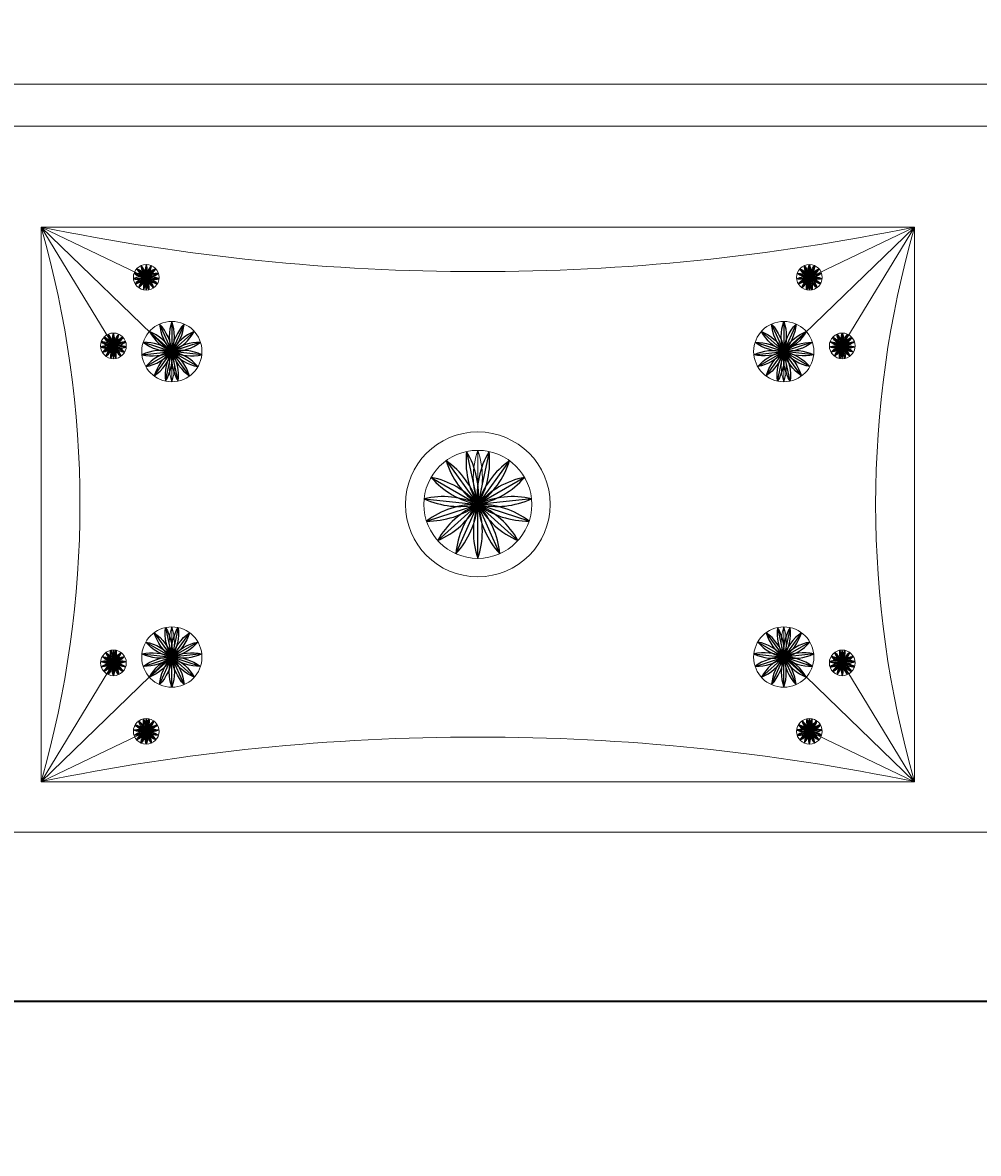
# Model space of a CAD drawing. Units: inches. Extents: x -61 to 1599, y -1316 to 257.
# Tile 5 of 204: x 123 to 149, y -1211 to -1180. Entities that reach past the tile are written whole.
import ezdxf

# ---------------------------------------------------------------- set-up
doc = ezdxf.new("R2010")
doc.units = ezdxf.units.IN
doc.header["$MEASUREMENT"] = 0
for name, color, linetype, lineweight in [('A-ANNO-DIMS', 2, 'Continuous', 18), ('FURNITURE', 83, 'Continuous', 18), ('WALLS', 4, 'Continuous', 35)]:
    doc.layers.add(name, color=color, linetype=linetype, lineweight=lineweight)
doc.layers.add('LT', color=8, linetype='Continuous')
doc.styles.get("Standard").update_dxf_attribs({"font": 'arial.ttf'})
doc.dimstyles.get("Standard").update_dxf_attribs({"dimtxt": 0.18, "dimasz": 0.18, "dimexe": 0.18, "dimexo": 0.0625, "dimgap": 0.09, "dimtad": 0, "dimtih": 1, "dimtoh": 1, "dimdec": 0, "dimzin": 0, "dimdsep": 46, "dimlunit": 3, "dimtxsty": 'Standard', "dimcen": 0.09, "dimadec": 0, "dimazin": 0, "dimtfac": 1, "dimtdec": 0, "dimtofl": 0, "dimtmove": 0, "dimatfit": 3, "dimfxl": 1, "dimtolj": 1, "dimtzin": 0, "dimarcsym": 0})

# ---------------------------------------------------------------- blocks, each defined once
blk = doc.blocks.new('*U15')
at = {"layer": 'LT'}
blk.add_line((0, 0.175), (0, -0.175), dxfattribs=at)
for centre, start, end in [((0.509, 0), 160.9983, 199.0017), ((-0.509, 0), 340.9983, 19.0017)]:
    blk.add_arc(centre, 0.539, start, end, dxfattribs=at)
blk = doc.blocks.new('*U16')
at = {"layer": 'LT', "transparency": 16777216}
for p, rotation in [((-66.605, -18.692), 48.00000000000001), ((-66.546, -18.649), 24), ((-66.404, -18.649), 336.0000000000001), ((-66.345, -18.692), 312), ((-66.649, -18.828), 96), ((-66.642, -18.755), 72), ((-66.627, -18.897), 120), ((-66.578, -18.951), 144), ((-66.512, -18.981), 168.0000000000001), ((-66.439, -18.981), 192), ((-66.372, -18.951), 216), ((-66.323, -18.897), 240), ((-66.308, -18.755), 288.0000000000001), ((-66.301, -18.828), 264)]:
    blk.add_blockref('*U15', p, dxfattribs=dict(at, rotation=rotation))
blk.add_blockref('*U15', (-66.475, -18.634), dxfattribs=at)
blk = doc.blocks.new('*U45')
at = {"layer": 'LT'}
blk.add_line((0, 0.175), (0, -0.175), dxfattribs=at)
for centre, start, end in [((0.509, 0), 160.9983, 199.0017), ((-0.509, 0), 340.9983, 19.0017)]:
    blk.add_arc(centre, 0.539, start, end, dxfattribs=at)
blk = doc.blocks.new('*U46')
at = {"layer": 'LT', "transparency": 16777216}
for p, rotation in [((-66.605, -18.692), 48.00000000000001), ((-66.546, -18.649), 24), ((-66.404, -18.649), 336.0000000000001), ((-66.345, -18.692), 312), ((-66.649, -18.828), 96), ((-66.642, -18.755), 72), ((-66.627, -18.897), 120), ((-66.578, -18.951), 144), ((-66.512, -18.981), 168.0000000000001), ((-66.439, -18.981), 192), ((-66.372, -18.951), 216), ((-66.323, -18.897), 240), ((-66.308, -18.755), 288.0000000000001), ((-66.301, -18.828), 264)]:
    blk.add_blockref('*U45', p, dxfattribs=dict(at, rotation=rotation))
blk.add_blockref('*U45', (-66.475, -18.634), dxfattribs=at)
blk = doc.blocks.new('*U9')
at = {"layer": 'LT'}
blk.add_line((0, 0.175), (0, -0.175), dxfattribs=at)
for centre, start, end in [((0.509, 0), 160.9983, 199.0017), ((-0.509, 0), 340.9983, 19.0017)]:
    blk.add_arc(centre, 0.539, start, end, dxfattribs=at)
blk = doc.blocks.new('*U10')
at = {"layer": 'LT', "transparency": 16777216}
for p, rotation in [((-66.605, -18.692), 48.00000000000001), ((-66.546, -18.649), 24), ((-66.404, -18.649), 336.0000000000001), ((-66.345, -18.692), 312), ((-66.649, -18.828), 96), ((-66.642, -18.755), 72), ((-66.627, -18.897), 120), ((-66.578, -18.951), 144), ((-66.512, -18.981), 168.0000000000001), ((-66.439, -18.981), 192), ((-66.372, -18.951), 216), ((-66.323, -18.897), 240), ((-66.308, -18.755), 288.0000000000001), ((-66.301, -18.828), 264)]:
    blk.add_blockref('*U9', p, dxfattribs=dict(at, rotation=rotation))
blk.add_blockref('*U9', (-66.475, -18.634), dxfattribs=at)
blk = doc.blocks.new('*U39')
at = {"layer": 'LT'}
blk.add_line((0, 0.175), (0, -0.175), dxfattribs=at)
for centre, start, end in [((0.509, 0), 160.9983, 199.0017), ((-0.509, 0), 340.9983, 19.0017)]:
    blk.add_arc(centre, 0.539, start, end, dxfattribs=at)
blk = doc.blocks.new('*U40')
at = {"layer": 'LT', "transparency": 16777216}
for p, rotation in [((-66.605, -18.692), 48.00000000000001), ((-66.546, -18.649), 24), ((-66.404, -18.649), 336.0000000000001), ((-66.345, -18.692), 312), ((-66.649, -18.828), 96), ((-66.642, -18.755), 72), ((-66.627, -18.897), 120), ((-66.578, -18.951), 144), ((-66.512, -18.981), 168.0000000000001), ((-66.439, -18.981), 192), ((-66.372, -18.951), 216), ((-66.323, -18.897), 240), ((-66.308, -18.755), 288.0000000000001), ((-66.301, -18.828), 264)]:
    blk.add_blockref('*U39', p, dxfattribs=dict(at, rotation=rotation))
blk.add_blockref('*U39', (-66.475, -18.634), dxfattribs=at)
blk = doc.blocks.new('*U17')
at = {"layer": 'LT'}
blk.add_line((0, 0.412), (0, -0.412), dxfattribs=at)
for centre, start, end in [((1.198, 0), 160.9983, 199.0017), ((-1.198, 0), 340.9983, 19.0017)]:
    blk.add_arc(centre, 1.267, start, end, dxfattribs=at)
blk = doc.blocks.new('*U18')
at = {"layer": 'LT', "transparency": 16777216}
for p, rotation in [((-156.501, -43.858), 24), ((-156.165, -43.858), 336.0000000000001), ((-156.725, -44.108), 72), ((-156.639, -43.959), 48.00000000000001), ((-156.027, -43.959), 312), ((-155.941, -44.108), 288.0000000000001), ((-156.743, -44.278), 96), ((-156.69, -44.441), 120), ((-156.575, -44.569), 144), ((-156.419, -44.639), 168), ((-156.247, -44.639), 192), ((-156.091, -44.569), 216), ((-155.976, -44.441), 240), ((-155.923, -44.278), 264)]:
    blk.add_blockref('*U17', p, dxfattribs=dict(at, rotation=rotation))
blk.add_blockref('*U17', (-156.333, -43.823), dxfattribs=at)
blk = doc.blocks.new('*U33')
at = {"layer": 'LT'}
blk.add_line((0, 0.412), (0, -0.412), dxfattribs=at)
for centre, start, end in [((1.198, 0), 160.9983, 199.0017), ((-1.198, 0), 340.9983, 19.0017)]:
    blk.add_arc(centre, 1.267, start, end, dxfattribs=at)
blk = doc.blocks.new('*U34')
at = {"layer": 'LT', "transparency": 16777216}
for p, rotation in [((-156.501, -43.858), 24), ((-156.165, -43.858), 336.0000000000001), ((-156.725, -44.108), 72), ((-156.639, -43.959), 48.00000000000001), ((-156.027, -43.959), 312), ((-155.941, -44.108), 288.0000000000001), ((-156.743, -44.278), 96), ((-156.69, -44.441), 120), ((-156.575, -44.569), 144), ((-156.419, -44.639), 168), ((-156.247, -44.639), 192), ((-156.091, -44.569), 216), ((-155.976, -44.441), 240), ((-155.923, -44.278), 264)]:
    blk.add_blockref('*U33', p, dxfattribs=dict(at, rotation=rotation))
blk.add_blockref('*U33', (-156.333, -43.823), dxfattribs=at)
blk = doc.blocks.new('*U11')
at = {"layer": 'LT'}
blk.add_line((0, 0.739), (0, -0.739), dxfattribs=at)
for centre, start, end in [((2.147, 0), 160.9983, 199.0017), ((-2.147, 0), 340.9983, 19.0017)]:
    blk.add_arc(centre, 2.27, start, end, dxfattribs=at)
blk = doc.blocks.new('*U12')
at = {"layer": 'LT', "transparency": 16777216}
for p, rotation in [((-280.542, -78.621), 23.99999999999999), ((-279.941, -78.621), 336.0000000000001), ((-280.791, -78.801), 48.00000000000001), ((-279.692, -78.801), 312), ((-280.945, -79.067), 72), ((-279.539, -79.067), 288.0000000000001), ((-280.977, -79.373), 96), ((-280.882, -79.665), 120), ((-279.602, -79.665), 240), ((-279.507, -79.373), 264), ((-280.676, -79.894), 144), ((-280.395, -80.019), 168), ((-280.088, -80.019), 191.9999999999999), ((-279.807, -79.894), 216)]:
    blk.add_blockref('*U11', p, dxfattribs=dict(at, rotation=rotation))
blk.add_blockref('*U11', (-280.242, -78.557), dxfattribs=at)
blk = doc.blocks.new('*U28')
at = {"layer": 'LT'}
blk.add_line((0, 0.412), (0, -0.412), dxfattribs=at)
for centre, start, end in [((1.198, 0), 160.9983, 199.0017), ((-1.198, 0), 340.9983, 19.0017)]:
    blk.add_arc(centre, 1.267, start, end, dxfattribs=at)
blk = doc.blocks.new('*U44')
at = {"layer": 'LT', "transparency": 16777216}
for p, rotation in [((-156.501, -43.858), 24), ((-156.165, -43.858), 336.0000000000001), ((-156.725, -44.108), 72), ((-156.639, -43.959), 48.00000000000001), ((-156.027, -43.959), 312), ((-155.941, -44.108), 288.0000000000001), ((-156.743, -44.278), 96), ((-156.69, -44.441), 120), ((-156.575, -44.569), 144), ((-156.419, -44.639), 168), ((-156.247, -44.639), 192), ((-156.091, -44.569), 216), ((-155.976, -44.441), 240), ((-155.923, -44.278), 264)]:
    blk.add_blockref('*U28', p, dxfattribs=dict(at, rotation=rotation))
blk.add_blockref('*U28', (-156.333, -43.823), dxfattribs=at)
blk = doc.blocks.new('*U13')
at = {"layer": 'LT'}
blk.add_line((0, 0.412), (0, -0.412), dxfattribs=at)
for centre, start, end in [((1.198, 0), 160.9983, 199.0017), ((-1.198, 0), 340.9983, 19.0017)]:
    blk.add_arc(centre, 1.267, start, end, dxfattribs=at)
blk = doc.blocks.new('*U14')
at = {"layer": 'LT', "transparency": 16777216}
for p, rotation in [((-156.501, -43.858), 24), ((-156.165, -43.858), 336.0000000000001), ((-156.725, -44.108), 72), ((-156.639, -43.959), 48.00000000000001), ((-156.027, -43.959), 312), ((-155.941, -44.108), 288.0000000000001), ((-156.743, -44.278), 96), ((-156.69, -44.441), 120), ((-156.575, -44.569), 144), ((-156.419, -44.639), 168), ((-156.247, -44.639), 192), ((-156.091, -44.569), 216), ((-155.976, -44.441), 240), ((-155.923, -44.278), 264)]:
    blk.add_blockref('*U13', p, dxfattribs=dict(at, rotation=rotation))
blk.add_blockref('*U13', (-156.333, -43.823), dxfattribs=at)
blk = doc.blocks.new('*U19')
at = {"layer": 'LT'}
blk.add_line((0, 0.175), (0, -0.175), dxfattribs=at)
for centre, start, end in [((0.509, 0), 160.9983, 199.0017), ((-0.509, 0), 340.9983, 19.0017)]:
    blk.add_arc(centre, 0.539, start, end, dxfattribs=at)
blk = doc.blocks.new('*U6')
at = {"layer": 'LT', "transparency": 16777216}
for p, rotation in [((-66.605, -18.692), 48.00000000000001), ((-66.546, -18.649), 24), ((-66.404, -18.649), 336.0000000000001), ((-66.345, -18.692), 312), ((-66.649, -18.828), 96), ((-66.642, -18.755), 72), ((-66.627, -18.897), 120), ((-66.578, -18.951), 144), ((-66.512, -18.981), 168.0000000000001), ((-66.439, -18.981), 192), ((-66.372, -18.951), 216), ((-66.323, -18.897), 240), ((-66.308, -18.755), 288.0000000000001), ((-66.301, -18.828), 264)]:
    blk.add_blockref('*U19', p, dxfattribs=dict(at, rotation=rotation))
blk.add_blockref('*U19', (-66.475, -18.634), dxfattribs=at)
blk = doc.blocks.new('*U35')
at = {"layer": 'LT'}
blk.add_line((0, 0.175), (0, -0.175), dxfattribs=at)
for centre, start, end in [((0.509, 0), 160.9983, 199.0017), ((-0.509, 0), 340.9983, 19.0017)]:
    blk.add_arc(centre, 0.539, start, end, dxfattribs=at)
blk = doc.blocks.new('*U36')
at = {"layer": 'LT', "transparency": 16777216}
for p, rotation in [((-66.605, -18.692), 48.00000000000001), ((-66.546, -18.649), 24), ((-66.404, -18.649), 336.0000000000001), ((-66.345, -18.692), 312), ((-66.649, -18.828), 96), ((-66.642, -18.755), 72), ((-66.627, -18.897), 120), ((-66.578, -18.951), 144), ((-66.512, -18.981), 168.0000000000001), ((-66.439, -18.981), 192), ((-66.372, -18.951), 216), ((-66.323, -18.897), 240), ((-66.308, -18.755), 288.0000000000001), ((-66.301, -18.828), 264)]:
    blk.add_blockref('*U35', p, dxfattribs=dict(at, rotation=rotation))
blk.add_blockref('*U35', (-66.475, -18.634), dxfattribs=at)
blk = doc.blocks.new('*U7')
at = {"layer": 'LT'}
blk.add_line((0, 0.175), (0, -0.175), dxfattribs=at)
for centre, start, end in [((0.509, 0), 160.9983, 199.0017), ((-0.509, 0), 340.9983, 19.0017)]:
    blk.add_arc(centre, 0.539, start, end, dxfattribs=at)
blk = doc.blocks.new('*U8')
at = {"layer": 'LT', "transparency": 16777216}
for p, rotation in [((-66.605, -18.692), 48.00000000000001), ((-66.546, -18.649), 24), ((-66.404, -18.649), 336.0000000000001), ((-66.345, -18.692), 312), ((-66.649, -18.828), 96), ((-66.642, -18.755), 72), ((-66.627, -18.897), 120), ((-66.578, -18.951), 144), ((-66.512, -18.981), 168.0000000000001), ((-66.439, -18.981), 192), ((-66.372, -18.951), 216), ((-66.323, -18.897), 240), ((-66.308, -18.755), 288.0000000000001), ((-66.301, -18.828), 264)]:
    blk.add_blockref('*U7', p, dxfattribs=dict(at, rotation=rotation))
blk.add_blockref('*U7', (-66.475, -18.634), dxfattribs=at)
blk = doc.blocks.new('*U37')
at = {"layer": 'LT'}
blk.add_line((0, 0.175), (0, -0.175), dxfattribs=at)
for centre, start, end in [((0.509, 0), 160.9983, 199.0017), ((-0.509, 0), 340.9983, 19.0017)]:
    blk.add_arc(centre, 0.539, start, end, dxfattribs=at)
blk = doc.blocks.new('*U38')
at = {"layer": 'LT', "transparency": 16777216}
for p, rotation in [((-66.605, -18.692), 48.00000000000001), ((-66.546, -18.649), 24), ((-66.404, -18.649), 336.0000000000001), ((-66.345, -18.692), 312), ((-66.649, -18.828), 96), ((-66.642, -18.755), 72), ((-66.627, -18.897), 120), ((-66.578, -18.951), 144), ((-66.512, -18.981), 168.0000000000001), ((-66.439, -18.981), 192), ((-66.372, -18.951), 216), ((-66.323, -18.897), 240), ((-66.308, -18.755), 288.0000000000001), ((-66.301, -18.828), 264)]:
    blk.add_blockref('*U37', p, dxfattribs=dict(at, rotation=rotation))
blk.add_blockref('*U37', (-66.475, -18.634), dxfattribs=at)
blk = doc.blocks.new('BED-DOUBLE')
for p, q in [((1.272, 20.467), (70.263, 20.467)), ((1.272, 19.317), (70.263, 19.317)), ((10.471, 1.379), (10.471, 16.557)), ((34.388, 16.557), (10.471, 16.557)), ((10.471, 16.557), (13.35, 15.18)), ((10.471, 16.557), (14.039, 13.107)), ((10.471, 16.557), (12.454, 13.305)), ((34.388, 16.557), (30.82, 13.107)), ((34.388, 16.557), (31.508, 15.18)), ((34.388, 16.557), (32.405, 13.305)), ((13.35, 15.18), (13.35, 14.829)), ((31.508, 15.18), (31.508, 14.829)), ((12.454, 13.305), (12.454, 12.955)), ((14.052, 13.149), (14.052, 12.324)), ((30.806, 13.149), (30.806, 12.324)), ((32.405, 13.305), (32.405, 12.955)), ((22.429, 8.968), (22.429, 10.447)), ((14.052, 4.788), (14.052, 5.613)), ((30.806, 4.788), (30.806, 5.613)), ((12.454, 4.631), (12.454, 4.982)), ((32.405, 4.631), (32.405, 4.982)), ((10.471, 1.379), (14.039, 4.83)), ((34.388, 1.379), (30.82, 4.83)), ((10.471, 1.379), (12.454, 4.631)), ((34.388, 1.379), (32.405, 4.631)), ((13.35, 2.756), (13.35, 3.107)), ((31.508, 2.756), (31.508, 3.107)), ((10.471, 1.379), (13.35, 2.756)), ((34.388, 1.379), (31.508, 2.756)), ((34.388, 1.379), (34.388, 1.379))]:
    blk.add_line(p, q)
for points in [[(1.272, 88.537), (1.272, 3.449, 0.414214), (4.722, 0), (66.813, 0, 0.414214), (70.263, 3.449), (70.263, 88.537, 0.414214), (66.813, 91.987), (4.722, 91.987, 0.414214)], [(13.35, 15.18, 0.167358), (13.35, 14.829, 0.167358)], [(12.454, 13.305, 0.167358), (12.454, 12.955, 0.167358)], [(14.052, 13.149, 0.167358), (14.052, 12.324, 0.167358)], [(30.806, 12.324, 0.167358), (30.806, 13.149, 0.167358)], [(32.405, 12.955, 0.167358), (32.405, 13.305, 0.167358)], [(22.429, 8.968, 0.167358), (22.429, 10.447, 0.167358)], [(14.052, 5.613, 0.167358), (14.052, 4.788, 0.167358)], [(30.806, 4.788, 0.167358), (30.806, 5.613, 0.167358)], [(12.454, 4.982, 0.167358), (12.454, 4.631, 0.167358)], [(32.405, 4.631, 0.167358), (32.405, 4.982, 0.167358)], [(13.35, 3.107, 0.167358), (13.35, 2.756, 0.167358)], [(31.508, 2.756, 0.167358), (31.508, 3.107, 0.167358)]]:
    blk.add_lwpolyline(points, format="xyb", close=True)
blk.add_lwpolyline([(34.388, 16.557), (34.388, 1.379), (10.471, 1.379), (10.471, 16.557), (34.388, 16.557), (34.388, 1.379), (10.471, 1.379)])
for centre, radius in [((13.35, 15.18), 0.351), ((31.508, 15.18), 0.351), ((14.052, 13.149), 0.825), ((30.806, 13.149), 0.825), ((12.454, 13.305), 0.351), ((32.405, 13.305), 0.351), ((22.429, 8.968), 1.982), ((22.429, 8.968), 1.478), ((14.052, 4.788), 0.825), ((30.806, 4.788), 0.825), ((12.454, 4.631), 0.351), ((32.405, 4.631), 0.351), ((13.35, 2.756), 0.351), ((31.508, 2.756), 0.351)]:
    blk.add_circle(centre, radius)
for centre, radius, start, end in [((-16.003, 8.968), 27.54, 344.0046, 15.9954), ((22.429, 74.54), 59.203, 258.34678, 281.65322), ((60.861, 8.968), 27.54, 164.0046, 195.9954), ((32.017, 15.005), 0.539, 160.9983, 199.0017), ((30.999, 15.005), 0.539, 340.9983, 19.0017), ((22.429, -56.603), 59.203, 78.34678, 101.65322)]:
    blk.add_arc(centre, radius, start, end)
for name, p in [('*U40', (79.825, 33.99)), ('*U34', (170.385, 57.384)), ('*U46', (78.929, 32.115))]:
    blk.add_blockref(name, p)
at = {"extrusion": (0, 0, -1), "zscale": -1}
for name, p in [('*U36', (34.967, 33.99)), ('*U14', (125.527, 57.384)), ('*U38', (34.07, 32.115))]:
    blk.add_blockref(name, p, dxfattribs=at)
at = {"rotation": 180}
for name, p in [('*U12', (-257.812, -70.328)), ('*U44', (-125.527, -39.447)), ('*U8', (-34.07, -14.178)), ('*U6', (-34.967, -16.053))]:
    blk.add_blockref(name, p, dxfattribs=at)
at = {"extrusion": (0, 0, -1), "zscale": -1, "rotation": 180}
for name, p in [('*U18', (-170.385, -39.447)), ('*U16', (-78.929, -14.178)), ('*U10', (-79.825, -16.053))]:
    blk.add_blockref(name, p, dxfattribs=at)
blk = doc.blocks.new('*D635')
at = {"layer": 'A-ANNO-DIMS', "color": 0, "lineweight": -2, "transparency": 16777216}
for p, q in [((111.872, -1202.381), (111.872, -1216.391)), ((183.57, -1202.381), (183.57, -1216.391)), ((112.052, -1216.211), (147.193, -1216.211)), ((183.39, -1216.211), (148.248, -1216.211))]:
    blk.add_line(p, q, dxfattribs=at)
at = {"layer": 'A-ANNO-DIMS', "color": 0, "transparency": 16777216}
for points in [[(112.052, -1216.181), (112.052, -1216.241), (111.872, -1216.211)], [(183.39, -1216.181), (183.39, -1216.241), (183.57, -1216.211)]]:
    blk.add_solid(points, dxfattribs=at)
at = {"layer": 'DEFPOINTS', "color": 0, "transparency": 16777216}
for p in [(111.872, -1202.318), (183.57, -1202.318), (183.57, -1216.211)]:
    blk.add_point(p, dxfattribs=at)
at = {"layer": 'A-ANNO-DIMS', "color": 0, "transparency": 16777216, "insert": (147.721, -1216.211), "char_height": 0.18, "attachment_point": 5}
blk.add_mtext('\\A1;72 TYP.', dxfattribs=at)
blk = doc.blocks.new('*D687')
at = {"layer": 'A-ANNO-DIMS', "color": 0, "lineweight": -2, "transparency": 16777216}
for p, q in [((289.418, 181.677), (-61.077, 181.677)), ((-60.897, 181.497), (-60.897, -528.952)), ((-60.897, -1239.765), (-60.897, -529.316)), ((319.64, -1239.945), (-61.077, -1239.945))]:
    blk.add_line(p, q, dxfattribs=at)
at = {"layer": 'A-ANNO-DIMS', "color": 0, "transparency": 16777216}
for points in [[(-60.927, 181.497), (-60.867, 181.497), (-60.897, 181.677)], [(-60.927, -1239.765), (-60.867, -1239.765), (-60.897, -1239.945)]]:
    blk.add_solid(points, dxfattribs=at)
at = {"layer": 'DEFPOINTS', "color": 0, "transparency": 16777216}
for p in [(289.481, 181.677), (-60.897, -1239.945), (319.703, -1239.945)]:
    blk.add_point(p, dxfattribs=at)
at = {"layer": 'A-ANNO-DIMS', "color": 0, "transparency": 16777216, "insert": (-60.897, -529.134), "char_height": 0.18, "attachment_point": 5}
blk.add_mtext('\\A1;1421.6', dxfattribs=at)

msp = doc.modelspace()

# ---------------------------------------------------------------- linework, layer by layer
at = {"layer": 'WALLS'}
msp.add_line((14.7028, -1206.9446), (237.7028, -1206.9446), dxfattribs=at)

# ---------------------------------------------------------------- block references
at = {"layer": 'FURNITURE'}
msp.add_blockref('BED-DOUBLE', (113.2612, -1202.3177), dxfattribs=at)

# ---------------------------------------------------------------- dimensions: what is measured, and where the dimension line sits
at = {"layer": 'A-ANNO-DIMS'}
dim = msp.add_linear_dim(base=(-60.8972, -1239.9446), p1=(289.4807, 181.6771), p2=(319.7028, -1239.9446), angle=90, dimstyle='Standard', override={"dimdec": 1, "dimlfac": 1, "dimrnd": 0, "dimzin": 0, "dimdsep": 46, "dimlunit": 2}, dxfattribs=at)
dim.commit()
dim.dimension.update_dxf_attribs({"geometry": '*D687', "text_midpoint": (-60.8972, -529.1337)})
dim = msp.add_linear_dim(base=(183.5695, -1216.2111), p1=(111.8719, -1202.3182), p2=(183.5695, -1202.3182), text='<> TYP.', dimstyle='Standard', override={"dimdec": 0, "dimlfac": 1, "dimrnd": 0, "dimzin": 0, "dimdsep": 46, "dimlunit": 2}, dxfattribs=at)
dim.commit()
dim.dimension.update_dxf_attribs({"geometry": '*D635', "text_midpoint": (147.7207, -1216.2111)})

doc.saveas('drawing.dxf')
